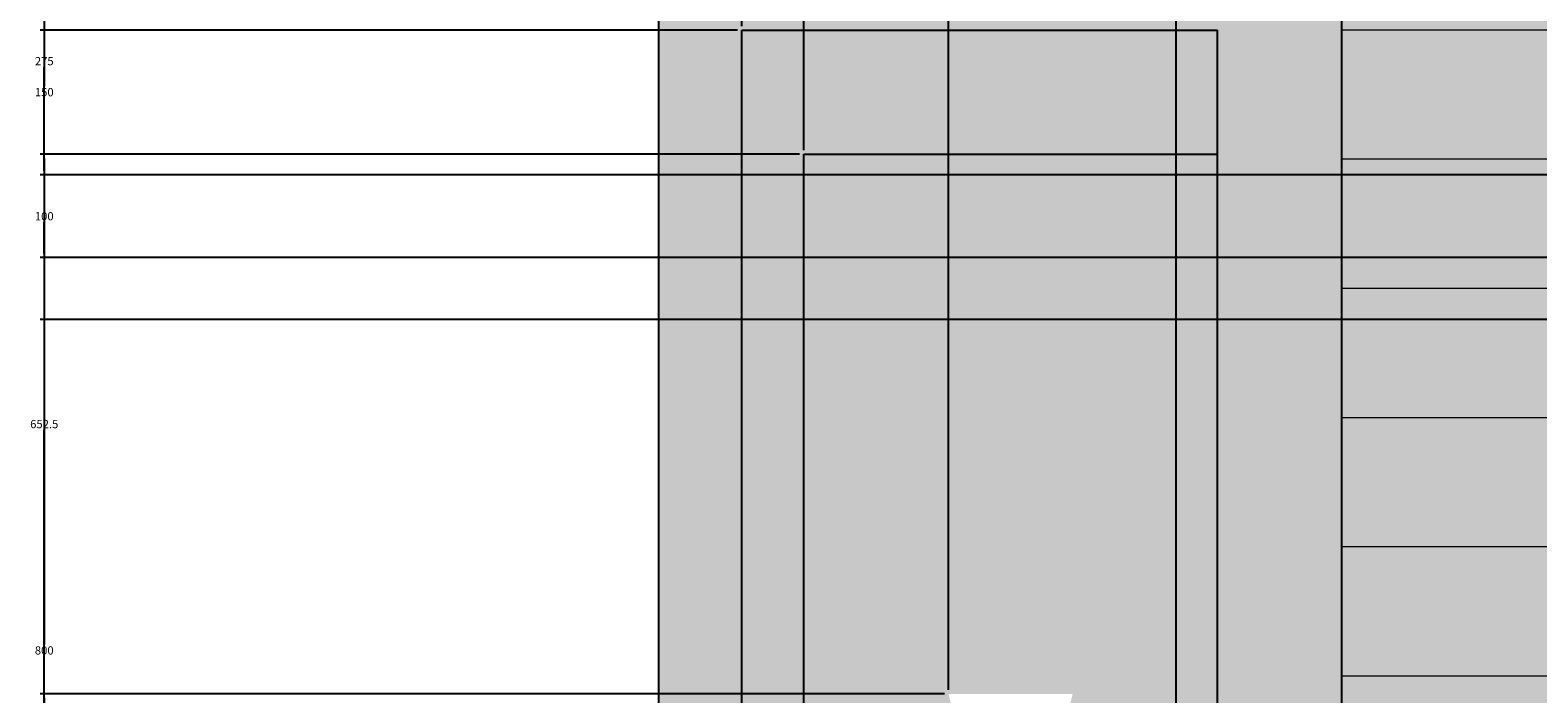
# Model space of a CAD drawing. Units: millimetres. Extents: x 2970 to 7764, y 2196 to 7505.
# Tile 7 of 13: x 2970 to 4793, y 5603 to 6406. Entities that reach past the tile are written whole.
import ezdxf

# ---------------------------------------------------------------- set-up
doc = ezdxf.new("R2010")
doc.units = ezdxf.units.MM
doc.header["$MEASUREMENT"] = 0
for name, color, linetype, lineweight in [('A-ANNO-DIMS', 2, 'Continuous', 18), ('A-ELEV', 7, 'Continuous', 25), ('A-ELEV-PATT', 8, 'Continuous', 13)]:
    doc.layers.add(name, color=color, linetype=linetype, lineweight=lineweight)
doc.styles.get("Standard").update_dxf_attribs({"font": 'arial.ttf'})
doc.dimstyles.get("Standard").update_dxf_attribs({"dimtxt": 10, "dimasz": 5, "dimexe": 5, "dimexo": 5, "dimgap": 2, "dimtad": 0, "dimtih": 1, "dimtoh": 1, "dimdec": 0, "dimzin": 0, "dimdsep": 46, "dimtxsty": 'Standard', "dimcen": 2, "dimadec": 0, "dimazin": 0, "dimtfac": 1, "dimtdec": 0, "dimtofl": 0, "dimtmove": 0, "dimatfit": 3, "dimfxl": 1, "dimtolj": 1, "dimtzin": 0, "dimarcsym": 0})

# ---------------------------------------------------------------- blocks, each defined once
blk = doc.blocks.new('*D12')
at = {"layer": 'A-ANNO-DIMS', "color": 0, "lineweight": -2, "transparency": 16777216}
for p, q in [((3830.5, 6410.8), (3830.5, 7503.8)), ((3835.5, 7498.8), (3858.8, 7498.8)), ((3900.5, 7498.8), (3877.2, 7498.8)), ((3905.5, 6260.8), (3905.5, 7503.8))]:
    blk.add_line(p, q, dxfattribs=at)
at = {"layer": 'A-ANNO-DIMS', "color": 0, "transparency": 16777216}
for points in [[(3835.5, 7499.6), (3835.5, 7498), (3830.5, 7498.8)], [(3900.5, 7499.6), (3900.5, 7498), (3905.5, 7498.8)]]:
    blk.add_solid(points, dxfattribs=at)
at = {"layer": 'Defpoints', "color": 0, "transparency": 16777216}
for p in [(3905.5, 7498.8), (3830.5, 6405.8), (3905.5, 6255.8)]:
    blk.add_point(p, dxfattribs=at)
at = {"layer": 'A-ANNO-DIMS', "color": 0, "transparency": 16777216, "insert": (3868, 7498.8), "char_height": 10, "attachment_point": 5}
blk.add_mtext('\\A1;75', dxfattribs=at)
blk = doc.blocks.new('*D13')
at = {"layer": 'A-ANNO-DIMS', "color": 0, "lineweight": -2, "transparency": 16777216}
for p, q in [((3905.5, 6260.8), (3905.5, 7503.8)), ((3910.5, 7498.8), (3980.4, 7498.8)), ((4075.5, 7498.8), (4005.6, 7498.8)), ((4080.5, 5608.3), (4080.5, 7503.8))]:
    blk.add_line(p, q, dxfattribs=at)
at = {"layer": 'A-ANNO-DIMS', "color": 0, "transparency": 16777216}
for points in [[(3910.5, 7499.6), (3910.5, 7498), (3905.5, 7498.8)], [(4075.5, 7499.6), (4075.5, 7498), (4080.5, 7498.8)]]:
    blk.add_solid(points, dxfattribs=at)
at = {"layer": 'Defpoints', "color": 0, "transparency": 16777216}
for p in [(4080.5, 7498.8), (3905.5, 6255.8), (4080.5, 5603.3)]:
    blk.add_point(p, dxfattribs=at)
at = {"layer": 'A-ANNO-DIMS', "color": 0, "transparency": 16777216, "insert": (3993, 7498.8), "char_height": 10, "attachment_point": 5}
blk.add_mtext('\\A1;175', dxfattribs=at)
blk = doc.blocks.new('*D14')
at = {"layer": 'A-ANNO-DIMS', "color": 0, "lineweight": -2, "transparency": 16777216}
for p, q in [((4080.5, 5608.3), (4080.5, 7503.8)), ((4085.5, 7498.8), (4179.8, 7498.8)), ((4300.5, 7498.8), (4206.2, 7498.8)), ((4305.5, 7260.8), (4305.5, 7503.8))]:
    blk.add_line(p, q, dxfattribs=at)
at = {"layer": 'A-ANNO-DIMS', "color": 0, "transparency": 16777216}
for points in [[(4085.5, 7499.6), (4085.5, 7498), (4080.5, 7498.8)], [(4300.5, 7499.6), (4300.5, 7498), (4305.5, 7498.8)]]:
    blk.add_solid(points, dxfattribs=at)
at = {"layer": 'Defpoints', "color": 0, "transparency": 16777216}
for p in [(4305.5, 7498.8), (4305.5, 7255.8), (4080.5, 5603.3)]:
    blk.add_point(p, dxfattribs=at)
at = {"layer": 'A-ANNO-DIMS', "color": 0, "transparency": 16777216, "insert": (4193, 7498.8), "char_height": 10, "attachment_point": 5}
blk.add_mtext('\\A1;225', dxfattribs=at)
blk = doc.blocks.new('*D24')
at = {"layer": 'A-ANNO-DIMS', "color": 0, "lineweight": -2, "transparency": 16777216}
for p, q in [((4075.5, 5603.3), (2982.5, 5603.3)), ((2987.5, 5598.3), (2987.5, 5422.9)), ((2987.5, 5233.3), (2987.5, 5408.7)), ((4075.5, 5228.3), (2982.5, 5228.3))]:
    blk.add_line(p, q, dxfattribs=at)
at = {"layer": 'A-ANNO-DIMS', "color": 0, "transparency": 16777216}
for points in [[(2986.7, 5598.3), (2988.3, 5598.3), (2987.5, 5603.3)], [(2986.7, 5233.3), (2988.3, 5233.3), (2987.5, 5228.3)]]:
    blk.add_solid(points, dxfattribs=at)
at = {"layer": 'Defpoints', "color": 0, "transparency": 16777216}
for p in [(2987.5, 5603.3), (4080.5, 5603.3), (4080.5, 5228.3)]:
    blk.add_point(p, dxfattribs=at)
at = {"layer": 'A-ANNO-DIMS', "color": 0, "transparency": 16777216, "insert": (2987.5, 5415.8), "char_height": 10, "attachment_point": 5}
blk.add_mtext('\\A1;375', dxfattribs=at)
blk = doc.blocks.new('*D25')
at = {"layer": 'A-ANNO-DIMS', "color": 0, "lineweight": -2, "transparency": 16777216}
for p, q in [((3900.5, 6255.8), (2982.5, 6255.8)), ((2987.5, 6250.8), (2987.5, 5936.6)), ((2987.5, 5608.3), (2987.5, 5922.4)), ((4075.5, 5603.3), (2982.5, 5603.3))]:
    blk.add_line(p, q, dxfattribs=at)
at = {"layer": 'A-ANNO-DIMS', "color": 0, "transparency": 16777216}
for points in [[(2986.7, 6250.8), (2988.3, 6250.8), (2987.5, 6255.8)], [(2986.7, 5608.3), (2988.3, 5608.3), (2987.5, 5603.3)]]:
    blk.add_solid(points, dxfattribs=at)
at = {"layer": 'Defpoints', "color": 0, "transparency": 16777216}
for p in [(2987.5, 6255.8), (3905.5, 6255.8), (4080.5, 5603.3)]:
    blk.add_point(p, dxfattribs=at)
at = {"layer": 'A-ANNO-DIMS', "color": 0, "transparency": 16777216, "insert": (2987.5, 5929.5), "char_height": 10, "attachment_point": 5}
blk.add_mtext('\\A1;652.5', dxfattribs=at)
blk = doc.blocks.new('*D26')
at = {"layer": 'A-ANNO-DIMS', "color": 0, "lineweight": -2, "transparency": 16777216}
for p, q in [((3825.5, 6405.8), (2982.5, 6405.8)), ((2987.5, 6400.8), (2987.5, 6337.9)), ((2987.5, 6260.8), (2987.5, 6323.7)), ((3900.5, 6255.8), (2982.5, 6255.8))]:
    blk.add_line(p, q, dxfattribs=at)
at = {"layer": 'A-ANNO-DIMS', "color": 0, "transparency": 16777216}
for points in [[(2986.7, 6400.8), (2988.3, 6400.8), (2987.5, 6405.8)], [(2986.7, 6260.8), (2988.3, 6260.8), (2987.5, 6255.8)]]:
    blk.add_solid(points, dxfattribs=at)
at = {"layer": 'Defpoints', "color": 0, "transparency": 16777216}
for p in [(2987.5, 6405.8), (3830.5, 6405.8), (3905.5, 6255.8)]:
    blk.add_point(p, dxfattribs=at)
at = {"layer": 'A-ANNO-DIMS', "color": 0, "transparency": 16777216, "insert": (2987.5, 6330.8), "char_height": 10, "attachment_point": 5}
blk.add_mtext('\\A1;150', dxfattribs=at)
blk = doc.blocks.new('*D34')
at = {"layer": 'A-ANNO-DIMS', "color": 0, "lineweight": -2, "transparency": 16777216}
for p, q in [((4355.5, 4210.8), (4355.5, 7503.8)), ((4360.5, 7498.8), (4607.5, 7498.8)), ((4880.5, 7498.8), (4633.5, 7498.8)), ((4885.5, 4210.8), (4885.5, 7503.8))]:
    blk.add_line(p, q, dxfattribs=at)
at = {"layer": 'A-ANNO-DIMS', "color": 0, "transparency": 16777216}
for points in [[(4360.5, 7499.6), (4360.5, 7498), (4355.5, 7498.8)], [(4880.5, 7499.6), (4880.5, 7498), (4885.5, 7498.8)]]:
    blk.add_solid(points, dxfattribs=at)
at = {"layer": 'Defpoints', "color": 0, "transparency": 16777216}
for p in [(4885.5, 7498.8), (4355.5, 4205.8), (4885.5, 4205.8)]:
    blk.add_point(p, dxfattribs=at)
at = {"layer": 'A-ANNO-DIMS', "color": 0, "transparency": 16777216, "insert": (4620.5, 7498.8), "char_height": 10, "attachment_point": 5}
blk.add_mtext('\\A1;530', dxfattribs=at)
blk = doc.blocks.new('*D76')
at = {"layer": 'A-ANNO-DIMS', "color": 0, "lineweight": -2, "transparency": 16777216}
for p, q in [((6100.5, 6055.8), (2982.5, 6055.8)), ((2987.5, 6050.8), (2987.5, 5662.9)), ((2987.5, 5260.8), (2987.5, 5648.7)), ((6100.5, 5255.8), (2982.5, 5255.8))]:
    blk.add_line(p, q, dxfattribs=at)
at = {"layer": 'A-ANNO-DIMS', "color": 0, "transparency": 16777216}
for points in [[(2986.7, 6050.8), (2988.3, 6050.8), (2987.5, 6055.8)], [(2986.7, 5260.8), (2988.3, 5260.8), (2987.5, 5255.8)]]:
    blk.add_solid(points, dxfattribs=at)
at = {"layer": 'Defpoints', "color": 0, "transparency": 16777216}
for p in [(2987.5, 6055.8), (6105.5, 6055.8), (6105.5, 5255.8)]:
    blk.add_point(p, dxfattribs=at)
at = {"layer": 'A-ANNO-DIMS', "color": 0, "transparency": 16777216, "insert": (2987.5, 5655.8), "char_height": 10, "attachment_point": 5}
blk.add_mtext('\\A1;800', dxfattribs=at)
blk = doc.blocks.new('*D81')
at = {"layer": 'A-ANNO-DIMS', "color": 0, "lineweight": -2, "transparency": 16777216}
for p, q in [((6000.5, 6230.8), (2982.5, 6230.8)), ((2987.5, 6225.8), (2987.5, 6187.9)), ((2987.5, 6135.8), (2987.5, 6173.7)), ((6025.5, 6130.8), (2982.5, 6130.8))]:
    blk.add_line(p, q, dxfattribs=at)
at = {"layer": 'A-ANNO-DIMS', "color": 0, "transparency": 16777216}
for points in [[(2986.7, 6225.8), (2988.3, 6225.8), (2987.5, 6230.8)], [(2986.7, 6135.8), (2988.3, 6135.8), (2987.5, 6130.8)]]:
    blk.add_solid(points, dxfattribs=at)
at = {"layer": 'Defpoints', "color": 0, "transparency": 16777216}
for p in [(2987.5, 6230.8), (6005.5, 6230.8), (6030.5, 6130.8)]:
    blk.add_point(p, dxfattribs=at)
at = {"layer": 'A-ANNO-DIMS', "color": 0, "transparency": 16777216, "insert": (2987.5, 6180.8), "char_height": 10, "attachment_point": 5}
blk.add_mtext('\\A1;100', dxfattribs=at)
blk = doc.blocks.new('*D82')
at = {"layer": 'A-ANNO-DIMS', "color": 0, "lineweight": -2, "transparency": 16777216}
for p, q in [((6000.5, 6505.8), (2982.5, 6505.8)), ((2987.5, 6500.8), (2987.5, 6375.4)), ((2987.5, 6235.8), (2987.5, 6361.2)), ((6000.5, 6230.8), (2982.5, 6230.8))]:
    blk.add_line(p, q, dxfattribs=at)
at = {"layer": 'A-ANNO-DIMS', "color": 0, "transparency": 16777216}
for points in [[(2986.7, 6500.8), (2988.3, 6500.8), (2987.5, 6505.8)], [(2986.7, 6235.8), (2988.3, 6235.8), (2987.5, 6230.8)]]:
    blk.add_solid(points, dxfattribs=at)
at = {"layer": 'Defpoints', "color": 0, "transparency": 16777216}
for p in [(2987.5, 6505.8), (6005.5, 6505.8), (6005.5, 6230.8)]:
    blk.add_point(p, dxfattribs=at)
at = {"layer": 'A-ANNO-DIMS', "color": 0, "transparency": 16777216, "insert": (2987.5, 6368.3), "char_height": 10, "attachment_point": 5}
blk.add_mtext('\\A1;275', dxfattribs=at)

msp = doc.modelspace()

# ---------------------------------------------------------------- hatches: boundary and pattern name
at = {"layer": 'A-ELEV-PATT'}
h = msp.add_hatch(color=256, dxfattribs=at)
h.dxf.hatch_style = 1
h.paths.add_polyline_path([(6405.5, 7255.789), (4305.5, 7255.789), (4305.5, 6505.789), (3730.5, 6505.789), (3730.5, 4205.789), (3730.5, 2945.789), (3730.5, 2895.789), (3830.5, 2895.789), (3830.5, 4205.789), (3830.5, 6405.789), (4405.5, 6405.789), (4405.5, 4205.789), (6905.5, 4205.789), (6905.5, 2945.789), (6905.5, 2845.789), (7155.5, 2845.789), (7155.5, 2945.789), (7155.5, 4205.789), (7155.5, 4455.789), (4555.5, 4455.789), (4555.5, 6505.789), (4555.5, 7005.789), (6155.5, 7005.789), (6155.5, 6755.789), (6405.5, 6755.789)])
h.paths.add_polyline_path([(7405.5, 6755.789), (6155.5, 6755.789), (5755.5, 6755.789), (5755.5, 5005.789), (7405.5, 5005.789)])
h.paths.add_polyline_path([(7155.5, 6505.789), (7155.5, 5255.789), (6005.5, 5255.789), (6005.5, 6505.789)], flags=16)
h.paths.add_polyline_path([(6105.5, 5520.789), (6105.5, 6055.789), (6455.5, 6055.789), (6455.5, 5520.789), (6655.5, 5520.789), (6655.5, 5605.789), (6655.5, 5955.789), (6955.5, 5955.789), (6955.5, 5605.789), (6955.5, 5520.789)], flags=0)
h.paths.add_polyline_path([(6425.5, 5755.789), (6425.5, 5655.789), (6425.5, 5555.789), (6405.5, 5555.789), (6405.5, 5755.789)], flags=0)
h.paths.add_polyline_path([(6955.5, 5505.789), (6955.5, 5405.789), (6655.5, 5405.789), (6655.5, 5505.789)], flags=0)
h = msp.add_hatch(color=256, dxfattribs=at)
h.set_gradient(color1=(147, 149, 152), color2=(199, 200, 202), name='CURVED')
h.paths.add_polyline_path([(6955.5, 4455.789), (6955.5, 5005.789), (5755.5, 5005.789), (5755.5, 6755.789), (6155.5, 6755.789), (6155.5, 7005.789), (4555.5, 7005.789), (4555.5, 6505.789), (4555.5, 4455.789)])
h.paths.add_polyline_path([(5015.81, 5462.49), (5015.81, 6062.49), (5455.81, 6062.49), (5455.81, 5462.49)], flags=16)
h.paths.add_polyline_path([(5035.81, 5482.49), (5035.81, 6042.49), (5155.81, 6042.49), (5155.81, 5482.49)], flags=0)
h.paths.add_polyline_path([(5175.81, 5482.49), (5175.81, 6042.49), (5295.81, 6042.49), (5295.81, 5482.49)], flags=0)
h.paths.add_polyline_path([(5315.81, 5482.49), (5315.81, 6042.49), (5435.81, 6042.49), (5435.81, 5482.49)], flags=0)
h.paths.add_polyline_path([(4865.81, 6162.49), (4865.81, 6212.49), (4840.81, 6212.49), (4840.81, 6237.49), (5630.81, 6237.49), (5630.81, 6212.49), (5605.81, 6212.49), (5605.81, 6162.49), (5015.81, 6162.49)], flags=16)
h = msp.add_hatch(dxfattribs=at)
h.set_pattern_fill('ANSI31', color=256, scale=1250, angle=135, style=0)
h.paths.add_polyline_path([(5755.5, 6755.789), (6155.5, 6755.789), (6155.5, 7005.789), (4555.5, 7005.789), (4555.5, 6505.789), (4555.5, 4455.789), (6955.5, 4455.789), (6955.5, 5005.789), (5755.5, 5005.789)])
h.paths.add_polyline_path([(5015.81, 5462.49), (5015.81, 6062.49), (5455.81, 6062.49), (5455.81, 5462.49)], flags=16)
h.paths.add_polyline_path([(5035.81, 5482.49), (5035.81, 6042.49), (5155.81, 6042.49), (5155.81, 5482.49)], flags=0)
h.paths.add_polyline_path([(5175.81, 5482.49), (5175.81, 6042.49), (5295.81, 6042.49), (5295.81, 5482.49)], flags=0)
h.paths.add_polyline_path([(5315.81, 5482.49), (5315.81, 6042.49), (5435.81, 6042.49), (5435.81, 5482.49)], flags=0)
h.paths.add_polyline_path([(4865.81, 6162.49), (4865.81, 6212.49), (4840.81, 6212.49), (4840.81, 6237.49), (5630.81, 6237.49), (5630.81, 6212.49), (5605.81, 6212.49), (5605.81, 6162.49), (5015.81, 6162.49)], flags=16)
h = msp.add_hatch(color=256, dxfattribs=at)
h.set_gradient(color1=(76, 38, 38), color2=(99, 100, 102), name='INVSPHERICAL')
h.paths.add_polyline_path([(3830.5, 6405.789), (3830.5, 4205.789), (3830.5, 2895.789), (3905.5, 2895.789), (3905.5, 4205.789), (3905.5, 6255.789), (4405.5, 6255.789), (4405.5, 6405.789)])
h = msp.add_hatch(color=256, dxfattribs=at)
h.set_gradient(color1=(53, 53, 54), color2=(99, 100, 102), name='SPHERICAL')
h.paths.add_polyline_path([(4405.5, 6255.789), (3905.5, 6255.789), (3905.5, 4205.789), (3905.5, 2895.789), (4355.5, 2895.789), (4355.5, 2995.799, -0.50803883), (4340.162, 3038.75, -0.52056705), (4337.177, 3086.472, -0.19797947), (4355.5, 3108.072), (4355.5, 4205.789), (4405.5, 4205.789)])
h.paths.add_polyline_path([(4080.5, 5228.289), (4105.5, 5328.289), (4105.5, 5503.289), (4080.5, 5603.289), (4230.5, 5603.289), (4205.5, 5503.289), (4205.5, 5328.289), (4230.5, 5228.289)], flags=16)
h.paths.add_polyline_path([(4120.5, 5343.289), (4120.5, 5488.289), (4190.5, 5488.289), (4190.5, 5343.289)], flags=0)
h.paths.add_polyline_path([(4230.5, 3923.289), (4205.5, 3823.289), (4205.5, 3648.289), (4230.5, 3548.289), (4080.5, 3548.289), (4105.5, 3648.289), (4105.5, 3823.289), (4080.5, 3923.289)], flags=16)
h.paths.add_polyline_path([(4190.5, 3808.289), (4190.5, 3663.289), (4120.5, 3663.289), (4120.5, 3808.289)], flags=0)

# ---------------------------------------------------------------- linework, layer by layer
at = {"layer": 'A-ELEV'}
for p, q in [((3730.5, 4205.789), (3730.5, 6505.789)), ((4555.5, 6505.789), (4555.5, 4455.789)), ((3830.5, 4205.789), (3830.5, 6405.789)), ((3830.5, 6405.789), (4405.5, 6405.789)), ((4405.5, 4205.789), (4405.5, 6405.789)), ((3905.5, 6255.789), (4405.5, 6255.789)), ((3905.5, 4205.789), (3905.5, 6255.789))]:
    msp.add_line(p, q, dxfattribs=at)

# ---------------------------------------------------------------- dimensions: what is measured, and where the dimension line sits
at = {"layer": 'A-ANNO-DIMS'}
for base, p1, p2, picture, middle in [((3905.5, 7498.789), (3830.5, 6405.789), (3905.5, 6255.789), '*D12', (3868, 7498.789)), ((4080.5, 7498.789), (3905.5, 6255.789), (4080.5, 5603.289), '*D13', (3993, 7498.789)), ((4305.5, 7498.789), (4080.5, 5603.289), (4305.5, 7255.789), '*D14', (4193, 7498.789)), ((4885.5, 7498.789), (4355.5, 4205.789), (4885.5, 4205.789), '*D34', (4620.5, 7498.789))]:
    dim = msp.add_linear_dim(base=base, p1=p1, p2=p2, dimstyle='Standard', override={"dimdec": 0, "dimlfac": 1, "dimrnd": 0, "dimzin": 0, "dimdsep": 46, "dimlunit": 2}, dxfattribs=at)
    dim.commit()
    dim.dimension.update_dxf_attribs({"geometry": picture, "text_midpoint": middle})
for base, p1, p2, override, picture, middle in [((2987.5, 6505.789), (6005.5, 6230.789), (6005.5, 6505.789), {"dimdec": 0, "dimlfac": 1, "dimrnd": 0, "dimzin": 0, "dimdsep": 46, "dimlunit": 2}, '*D82', (2987.5, 6368.289)), ((2987.5, 6405.789), (3905.5, 6255.789), (3830.5, 6405.789), {"dimdec": 0, "dimlfac": 1, "dimrnd": 0, "dimzin": 0, "dimdsep": 46, "dimlunit": 2}, '*D26', (2987.5, 6330.789)), ((2987.5, 6255.789), (4080.5, 5603.289), (3905.5, 6255.789), {"dimdec": 1, "dimlfac": 1, "dimrnd": 0, "dimzin": 0, "dimdsep": 46, "dimlunit": 2}, '*D25', (2987.5, 5929.539)), ((2987.5, 6230.789), (6030.5, 6130.789), (6005.5, 6230.789), {"dimdec": 0, "dimlfac": 1, "dimrnd": 0, "dimzin": 0, "dimdsep": 46, "dimlunit": 2}, '*D81', (2987.5, 6180.789)), ((2987.5, 6055.789), (6105.5, 5255.789), (6105.5, 6055.789), {"dimdec": 0, "dimlfac": 1, "dimrnd": 0, "dimzin": 0, "dimdsep": 46, "dimlunit": 2}, '*D76', (2987.5, 5655.789)), ((2987.5, 5603.289), (4080.5, 5228.289), (4080.5, 5603.289), {"dimdec": 0, "dimlfac": 1, "dimrnd": 0, "dimzin": 0, "dimdsep": 46, "dimlunit": 2}, '*D24', (2987.5, 5415.789))]:
    dim = msp.add_linear_dim(base=base, p1=p1, p2=p2, angle=90, dimstyle='Standard', override=override, dxfattribs=at)
    dim.commit()
    dim.dimension.update_dxf_attribs({"geometry": picture, "text_midpoint": middle})

doc.saveas('drawing.dxf')
